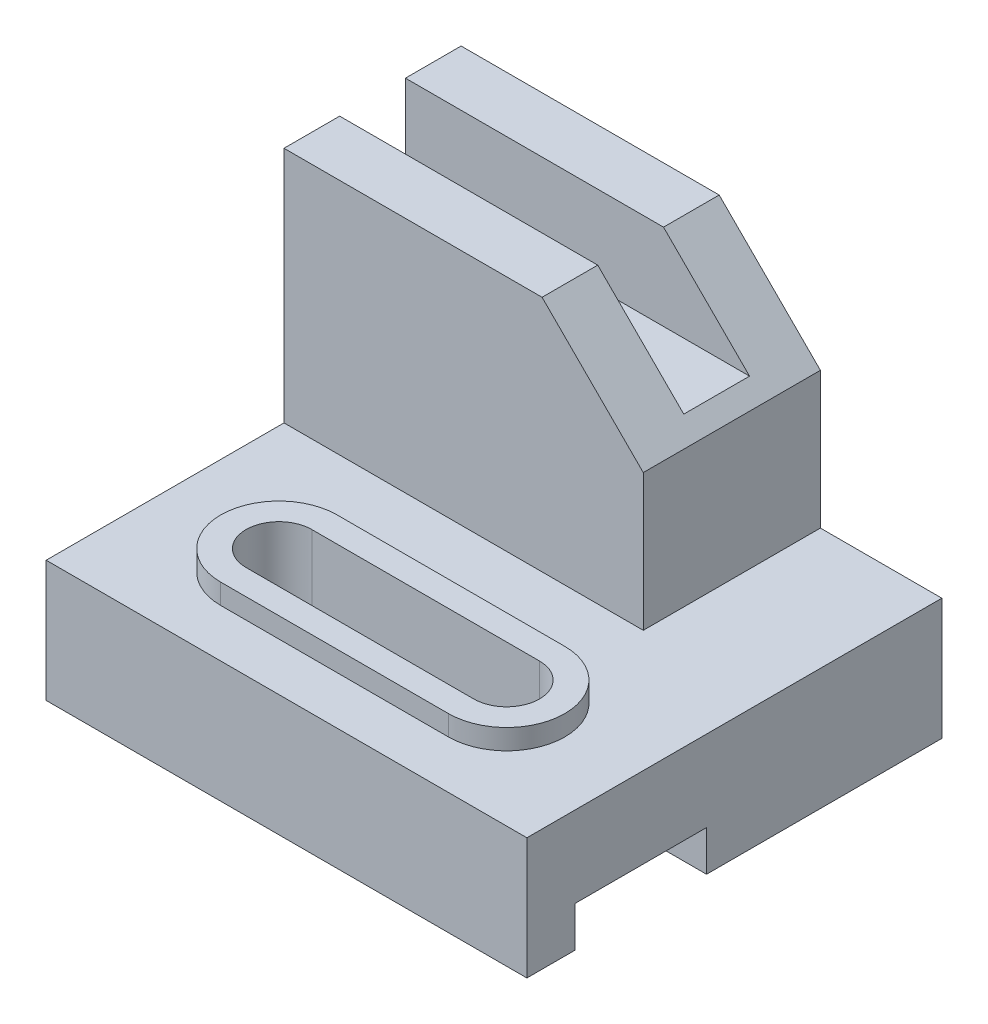
ISO-10303-21;
HEADER;
FILE_DESCRIPTION(('STEP AP214'),'2;1');
FILE_NAME('part.step','',(''),(''),'','','');
FILE_SCHEMA(('AUTOMOTIVE_DESIGN { 1 0 10303 214 1 1 1 1 }'));
ENDSEC;
DATA;
#1=APPLICATION_CONTEXT('core data for automotive mechanical design processes');
#2=APPLICATION_PROTOCOL_DEFINITION('international standard','automotive_design',2000,#1);
#3=PRODUCT_CONTEXT('',#1,'mechanical');
#4=PRODUCT('Part','Part','',(#3));
#5=PRODUCT_RELATED_PRODUCT_CATEGORY('part','',(#4));
#6=PRODUCT_DEFINITION_FORMATION('','',#4);
#7=PRODUCT_DEFINITION_CONTEXT('part definition',#1,'design');
#8=PRODUCT_DEFINITION('design','',#6,#7);
#9=PRODUCT_DEFINITION_SHAPE('','',#8);
#10=(LENGTH_UNIT() NAMED_UNIT(*) SI_UNIT(.MILLI.,.METRE.));
#11=(NAMED_UNIT(*) PLANE_ANGLE_UNIT() SI_UNIT($,.RADIAN.));
#12=(NAMED_UNIT(*) SI_UNIT($,.STERADIAN.) SOLID_ANGLE_UNIT());
#13=UNCERTAINTY_MEASURE_WITH_UNIT(LENGTH_MEASURE(1.E-05),#10,'distance_accuracy_value','');
#14=(GEOMETRIC_REPRESENTATION_CONTEXT(3) GLOBAL_UNCERTAINTY_ASSIGNED_CONTEXT((#13)) GLOBAL_UNIT_ASSIGNED_CONTEXT((#10,
#11,#12)) REPRESENTATION_CONTEXT('',''));
#15=CARTESIAN_POINT('',(0.,0.,0.));
#16=DIRECTION('',(0.,0.,1.));
#17=DIRECTION('',(1.,0.,0.));
#18=AXIS2_PLACEMENT_3D('',#15,#16,#17);
#19=CARTESIAN_POINT('',(95.,24.,0.));
#20=DIRECTION('',(0.,1.,0.));
#21=DIRECTION('',(0.,0.,1.));
#22=AXIS2_PLACEMENT_3D('',#19,#20,#21);
#23=PLANE('',#22);
#24=DIRECTION('',(0.,0.,-1.));
#25=VECTOR('',#24,1.);
#26=CARTESIAN_POINT('',(71.,24.,0.));
#27=LINE('',#26,#25);
#28=CARTESIAN_POINT('',(71.,24.,-47.));
#29=VERTEX_POINT('',#28);
#30=CARTESIAN_POINT('',(71.,24.,-82.));
#31=VERTEX_POINT('',#30);
#32=EDGE_CURVE('E345',#29,#31,#27,.T.);
#33=ORIENTED_EDGE('',*,*,#32,.F.);
#34=DIRECTION('',(-1.,0.,0.));
#35=VECTOR('',#34,1.);
#36=CARTESIAN_POINT('',(71.,24.,-47.));
#37=LINE('',#36,#35);
#38=CARTESIAN_POINT('',(0.,24.,-47.));
#39=VERTEX_POINT('',#38);
#40=EDGE_CURVE('E316',#29,#39,#37,.T.);
#41=ORIENTED_EDGE('',*,*,#40,.T.);
#42=DIRECTION('',(0.,0.,-1.));
#43=VECTOR('',#42,1.);
#44=CARTESIAN_POINT('',(0.,24.,0.));
#45=LINE('',#44,#43);
#46=CARTESIAN_POINT('',(0.,24.,0.));
#47=VERTEX_POINT('',#46);
#48=EDGE_CURVE('E279',#47,#39,#45,.T.);
#49=ORIENTED_EDGE('',*,*,#48,.F.);
#50=DIRECTION('',(-1.,0.,0.));
#51=VECTOR('',#50,1.);
#52=CARTESIAN_POINT('',(95.,24.,0.));
#53=LINE('',#52,#51);
#54=CARTESIAN_POINT('',(95.,24.,0.));
#55=VERTEX_POINT('',#54);
#56=EDGE_CURVE('E255',#55,#47,#53,.T.);
#57=ORIENTED_EDGE('',*,*,#56,.F.);
#58=DIRECTION('',(0.,0.,-1.));
#59=VECTOR('',#58,1.);
#60=CARTESIAN_POINT('',(95.,24.,0.));
#61=LINE('',#60,#59);
#62=CARTESIAN_POINT('',(95.,24.,-82.));
#63=VERTEX_POINT('',#62);
#64=EDGE_CURVE('E300',#55,#63,#61,.T.);
#65=ORIENTED_EDGE('',*,*,#64,.T.);
#66=DIRECTION('',(-1.,0.,0.));
#67=VECTOR('',#66,1.);
#68=CARTESIAN_POINT('',(95.,24.,-82.));
#69=LINE('',#68,#67);
#70=EDGE_CURVE('E253',#63,#31,#69,.T.);
#71=ORIENTED_EDGE('',*,*,#70,.T.);
#72=EDGE_LOOP('',(#33,#41,#49,#57,#65,#71));
#73=FACE_BOUND('',#72,.T.);
#74=DIRECTION('',(1.,0.,0.));
#75=VECTOR('',#74,1.);
#76=CARTESIAN_POINT('',(25.,24.,-9.5));
#77=LINE('',#76,#75);
#78=CARTESIAN_POINT('',(25.,24.,-9.5));
#79=VERTEX_POINT('',#78);
#80=CARTESIAN_POINT('',(70.,24.,-9.5));
#81=VERTEX_POINT('',#80);
#82=EDGE_CURVE('E362',#79,#81,#77,.T.);
#83=ORIENTED_EDGE('',*,*,#82,.F.);
#84=CARTESIAN_POINT('',(25.,24.,-21.));
#85=DIRECTION('',(0.,1.,0.));
#86=DIRECTION('',(0.,0.,1.));
#87=AXIS2_PLACEMENT_3D('',#84,#85,#86);
#88=CIRCLE('',#87,11.5);
#89=CARTESIAN_POINT('',(25.,24.,-32.5));
#90=VERTEX_POINT('',#89);
#91=EDGE_CURVE('E212',#90,#79,#88,.T.);
#92=ORIENTED_EDGE('',*,*,#91,.F.);
#93=DIRECTION('',(-1.,0.,0.));
#94=VECTOR('',#93,1.);
#95=CARTESIAN_POINT('',(25.,24.,-32.5));
#96=LINE('',#95,#94);
#97=CARTESIAN_POINT('',(70.,24.,-32.5));
#98=VERTEX_POINT('',#97);
#99=EDGE_CURVE('E359',#98,#90,#96,.T.);
#100=ORIENTED_EDGE('',*,*,#99,.F.);
#101=CARTESIAN_POINT('',(70.,24.,-21.));
#102=DIRECTION('',(0.,1.,0.));
#103=DIRECTION('',(0.,0.,1.));
#104=AXIS2_PLACEMENT_3D('',#101,#102,#103);
#105=CIRCLE('',#104,11.5);
#106=EDGE_CURVE('E356',#81,#98,#105,.T.);
#107=ORIENTED_EDGE('',*,*,#106,.F.);
#108=EDGE_LOOP('',(#83,#92,#100,#107));
#109=FACE_BOUND('',#108,.T.);
#110=ADVANCED_FACE('F43',(#73,#109),#23,.T.);
#111=CARTESIAN_POINT('',(95.,0.,-35.5));
#112=DIRECTION('',(0.,0.,1.));
#113=DIRECTION('',(1.,0.,0.));
#114=AXIS2_PLACEMENT_3D('',#111,#112,#113);
#115=PLANE('',#114);
#116=DIRECTION('',(0.,1.,0.));
#117=VECTOR('',#116,1.);
#118=CARTESIAN_POINT('',(0.,0.,-35.5));
#119=LINE('',#118,#117);
#120=CARTESIAN_POINT('',(0.,0.,-35.5));
#121=VERTEX_POINT('',#120);
#122=CARTESIAN_POINT('',(0.,8.,-35.5));
#123=VERTEX_POINT('',#122);
#124=EDGE_CURVE('E288',#121,#123,#119,.T.);
#125=ORIENTED_EDGE('',*,*,#124,.F.);
#126=DIRECTION('',(-1.,0.,0.));
#127=VECTOR('',#126,1.);
#128=CARTESIAN_POINT('',(95.,0.,-35.5));
#129=LINE('',#128,#127);
#130=CARTESIAN_POINT('',(95.,0.,-35.5));
#131=VERTEX_POINT('',#130);
#132=EDGE_CURVE('E248',#131,#121,#129,.T.);
#133=ORIENTED_EDGE('',*,*,#132,.F.);
#134=DIRECTION('',(0.,1.,0.));
#135=VECTOR('',#134,1.);
#136=CARTESIAN_POINT('',(95.,0.,-35.5));
#137=LINE('',#136,#135);
#138=CARTESIAN_POINT('',(95.,8.,-35.5));
#139=VERTEX_POINT('',#138);
#140=EDGE_CURVE('E269',#131,#139,#137,.T.);
#141=ORIENTED_EDGE('',*,*,#140,.T.);
#142=DIRECTION('',(-1.,0.,0.));
#143=VECTOR('',#142,1.);
#144=CARTESIAN_POINT('',(95.,8.,-35.5));
#145=LINE('',#144,#143);
#146=EDGE_CURVE('E262',#139,#123,#145,.T.);
#147=ORIENTED_EDGE('',*,*,#146,.T.);
#148=EDGE_LOOP('',(#125,#133,#141,#147));
#149=FACE_BOUND('',#148,.T.);
#150=ADVANCED_FACE('F400',(#149),#115,.T.);
#151=CARTESIAN_POINT('',(95.,0.,0.));
#152=DIRECTION('',(0.,1.,0.));
#153=DIRECTION('',(0.,0.,1.));
#154=AXIS2_PLACEMENT_3D('',#151,#152,#153);
#155=PLANE('',#154);
#156=DIRECTION('',(0.,0.,-1.));
#157=VECTOR('',#156,1.);
#158=CARTESIAN_POINT('',(0.,0.,0.));
#159=LINE('',#158,#157);
#160=CARTESIAN_POINT('',(0.,0.,-82.));
#161=VERTEX_POINT('',#160);
#162=EDGE_CURVE('E281',#121,#161,#159,.T.);
#163=ORIENTED_EDGE('',*,*,#162,.T.);
#164=DIRECTION('',(-1.,0.,0.));
#165=VECTOR('',#164,1.);
#166=CARTESIAN_POINT('',(95.,0.,-82.));
#167=LINE('',#166,#165);
#168=CARTESIAN_POINT('',(95.,0.,-82.));
#169=VERTEX_POINT('',#168);
#170=EDGE_CURVE('E247',#169,#161,#167,.T.);
#171=ORIENTED_EDGE('',*,*,#170,.F.);
#172=DIRECTION('',(0.,0.,-1.));
#173=VECTOR('',#172,1.);
#174=CARTESIAN_POINT('',(95.,0.,0.));
#175=LINE('',#174,#173);
#176=EDGE_CURVE('E302',#131,#169,#175,.T.);
#177=ORIENTED_EDGE('',*,*,#176,.F.);
#178=ORIENTED_EDGE('',*,*,#132,.T.);
#179=EDGE_LOOP('',(#163,#171,#177,#178));
#180=FACE_BOUND('',#179,.T.);
#181=ADVANCED_FACE('F409',(#180),#155,.F.);
#182=CARTESIAN_POINT('',(95.,0.,-82.));
#183=DIRECTION('',(0.,0.,1.));
#184=DIRECTION('',(1.,0.,0.));
#185=AXIS2_PLACEMENT_3D('',#182,#183,#184);
#186=PLANE('',#185);
#187=DIRECTION('',(-1.,0.,0.));
#188=VECTOR('',#187,1.);
#189=CARTESIAN_POINT('',(71.,71.,-82.));
#190=LINE('',#189,#188);
#191=CARTESIAN_POINT('',(50.9999999999999,71.,-82.));
#192=VERTEX_POINT('',#191);
#193=CARTESIAN_POINT('',(0.,71.,-82.));
#194=VERTEX_POINT('',#193);
#195=EDGE_CURVE('E317',#192,#194,#190,.T.);
#196=ORIENTED_EDGE('',*,*,#195,.F.);
#197=DIRECTION('',(0.707106781186548,-0.707106781186547,0.));
#198=VECTOR('',#197,1.);
#199=CARTESIAN_POINT('',(71.,51.,-82.));
#200=LINE('',#199,#198);
#201=CARTESIAN_POINT('',(71.,51.,-82.));
#202=VERTEX_POINT('',#201);
#203=EDGE_CURVE('E231',#192,#202,#200,.T.);
#204=ORIENTED_EDGE('',*,*,#203,.T.);
#205=DIRECTION('',(0.,1.,0.));
#206=VECTOR('',#205,1.);
#207=CARTESIAN_POINT('',(71.,0.,-82.));
#208=LINE('',#207,#206);
#209=EDGE_CURVE('E321',#31,#202,#208,.T.);
#210=ORIENTED_EDGE('',*,*,#209,.F.);
#211=ORIENTED_EDGE('',*,*,#70,.F.);
#212=DIRECTION('',(0.,1.,0.));
#213=VECTOR('',#212,1.);
#214=CARTESIAN_POINT('',(95.,0.,-82.));
#215=LINE('',#214,#213);
#216=EDGE_CURVE('E303',#169,#63,#215,.T.);
#217=ORIENTED_EDGE('',*,*,#216,.F.);
#218=ORIENTED_EDGE('',*,*,#170,.T.);
#219=DIRECTION('',(0.,1.,0.));
#220=VECTOR('',#219,1.);
#221=CARTESIAN_POINT('',(0.,0.,-82.));
#222=LINE('',#221,#220);
#223=EDGE_CURVE('E282',#161,#194,#222,.T.);
#224=ORIENTED_EDGE('',*,*,#223,.T.);
#225=EDGE_LOOP('',(#196,#204,#210,#211,#217,#218,#224));
#226=FACE_BOUND('',#225,.T.);
#227=ADVANCED_FACE('F411',(#226),#186,.F.);
#228=CARTESIAN_POINT('',(95.,0.,0.));
#229=DIRECTION('',(0.,0.,1.));
#230=DIRECTION('',(1.,0.,0.));
#231=AXIS2_PLACEMENT_3D('',#228,#229,#230);
#232=PLANE('',#231);
#233=DIRECTION('',(0.,1.,0.));
#234=VECTOR('',#233,1.);
#235=CARTESIAN_POINT('',(0.,0.,0.));
#236=LINE('',#235,#234);
#237=CARTESIAN_POINT('',(0.,0.,0.));
#238=VERTEX_POINT('',#237);
#239=EDGE_CURVE('E274',#238,#47,#236,.T.);
#240=ORIENTED_EDGE('',*,*,#239,.F.);
#241=DIRECTION('',(-1.,0.,0.));
#242=VECTOR('',#241,1.);
#243=CARTESIAN_POINT('',(95.,0.,0.));
#244=LINE('',#243,#242);
#245=CARTESIAN_POINT('',(95.,0.,0.));
#246=VERTEX_POINT('',#245);
#247=EDGE_CURVE('E258',#246,#238,#244,.T.);
#248=ORIENTED_EDGE('',*,*,#247,.F.);
#249=DIRECTION('',(0.,1.,0.));
#250=VECTOR('',#249,1.);
#251=CARTESIAN_POINT('',(95.,0.,0.));
#252=LINE('',#251,#250);
#253=EDGE_CURVE('E293',#246,#55,#252,.T.);
#254=ORIENTED_EDGE('',*,*,#253,.T.);
#255=ORIENTED_EDGE('',*,*,#56,.T.);
#256=EDGE_LOOP('',(#240,#248,#254,#255));
#257=FACE_BOUND('',#256,.T.);
#258=ADVANCED_FACE('F412',(#257),#232,.T.);
#259=CARTESIAN_POINT('',(95.,0.,0.));
#260=DIRECTION('',(0.,1.,0.));
#261=DIRECTION('',(0.,0.,1.));
#262=AXIS2_PLACEMENT_3D('',#259,#260,#261);
#263=PLANE('',#262);
#264=DIRECTION('',(0.,0.,-1.));
#265=VECTOR('',#264,1.);
#266=CARTESIAN_POINT('',(0.,0.,0.));
#267=LINE('',#266,#265);
#268=CARTESIAN_POINT('',(0.,0.,-9.5));
#269=VERTEX_POINT('',#268);
#270=EDGE_CURVE('E272',#238,#269,#267,.T.);
#271=ORIENTED_EDGE('',*,*,#270,.T.);
#272=DIRECTION('',(-1.,0.,0.));
#273=VECTOR('',#272,1.);
#274=CARTESIAN_POINT('',(95.,0.,-9.5));
#275=LINE('',#274,#273);
#276=CARTESIAN_POINT('',(95.,0.,-9.5));
#277=VERTEX_POINT('',#276);
#278=EDGE_CURVE('E256',#277,#269,#275,.T.);
#279=ORIENTED_EDGE('',*,*,#278,.F.);
#280=DIRECTION('',(0.,0.,-1.));
#281=VECTOR('',#280,1.);
#282=CARTESIAN_POINT('',(95.,0.,0.));
#283=LINE('',#282,#281);
#284=EDGE_CURVE('E291',#246,#277,#283,.T.);
#285=ORIENTED_EDGE('',*,*,#284,.F.);
#286=ORIENTED_EDGE('',*,*,#247,.T.);
#287=EDGE_LOOP('',(#271,#279,#285,#286));
#288=FACE_BOUND('',#287,.T.);
#289=ADVANCED_FACE('F471',(#288),#263,.F.);
#290=CARTESIAN_POINT('',(95.,0.,-9.5));
#291=DIRECTION('',(0.,0.,1.));
#292=DIRECTION('',(1.,0.,0.));
#293=AXIS2_PLACEMENT_3D('',#290,#291,#292);
#294=PLANE('',#293);
#295=DIRECTION('',(0.,1.,0.));
#296=VECTOR('',#295,1.);
#297=CARTESIAN_POINT('',(0.,0.,-9.5));
#298=LINE('',#297,#296);
#299=CARTESIAN_POINT('',(0.,8.,-9.5));
#300=VERTEX_POINT('',#299);
#301=EDGE_CURVE('E271',#269,#300,#298,.T.);
#302=ORIENTED_EDGE('',*,*,#301,.T.);
#303=DIRECTION('',(-1.,0.,0.));
#304=VECTOR('',#303,1.);
#305=CARTESIAN_POINT('',(95.,8.,-9.5));
#306=LINE('',#305,#304);
#307=CARTESIAN_POINT('',(95.,8.,-9.5));
#308=VERTEX_POINT('',#307);
#309=EDGE_CURVE('E261',#308,#300,#306,.T.);
#310=ORIENTED_EDGE('',*,*,#309,.F.);
#311=DIRECTION('',(0.,1.,0.));
#312=VECTOR('',#311,1.);
#313=CARTESIAN_POINT('',(95.,0.,-9.5));
#314=LINE('',#313,#312);
#315=EDGE_CURVE('E292',#277,#308,#314,.T.);
#316=ORIENTED_EDGE('',*,*,#315,.F.);
#317=ORIENTED_EDGE('',*,*,#278,.T.);
#318=EDGE_LOOP('',(#302,#310,#316,#317));
#319=FACE_BOUND('',#318,.T.);
#320=ADVANCED_FACE('F466',(#319),#294,.F.);
#321=CARTESIAN_POINT('',(95.,8.,0.));
#322=DIRECTION('',(0.,1.,0.));
#323=DIRECTION('',(0.,0.,1.));
#324=AXIS2_PLACEMENT_3D('',#321,#322,#323);
#325=PLANE('',#324);
#326=DIRECTION('',(-1.,0.,0.));
#327=VECTOR('',#326,1.);
#328=CARTESIAN_POINT('',(95.,8.,-27.5));
#329=LINE('',#328,#327);
#330=CARTESIAN_POINT('',(70.,8.00000000000001,-27.5));
#331=VERTEX_POINT('',#330);
#332=CARTESIAN_POINT('',(25.,8.00000000000001,-27.5));
#333=VERTEX_POINT('',#332);
#334=EDGE_CURVE('E55',#331,#333,#329,.T.);
#335=ORIENTED_EDGE('',*,*,#334,.T.);
#336=CARTESIAN_POINT('',(25.,8.00000000000001,-21.));
#337=DIRECTION('',(0.,1.,0.));
#338=DIRECTION('',(0.,0.,1.));
#339=AXIS2_PLACEMENT_3D('',#336,#337,#338);
#340=CIRCLE('',#339,6.5);
#341=CARTESIAN_POINT('',(25.,8.00000000000001,-14.5));
#342=VERTEX_POINT('',#341);
#343=EDGE_CURVE('E11',#333,#342,#340,.T.);
#344=ORIENTED_EDGE('',*,*,#343,.T.);
#345=DIRECTION('',(1.,0.,0.));
#346=VECTOR('',#345,1.);
#347=CARTESIAN_POINT('',(95.,8.,-14.5));
#348=LINE('',#347,#346);
#349=CARTESIAN_POINT('',(70.,8.,-14.5));
#350=VERTEX_POINT('',#349);
#351=EDGE_CURVE('E220',#342,#350,#348,.T.);
#352=ORIENTED_EDGE('',*,*,#351,.T.);
#353=CARTESIAN_POINT('',(70.,8.00000000000001,-21.));
#354=DIRECTION('',(0.,1.,0.));
#355=DIRECTION('',(0.,0.,1.));
#356=AXIS2_PLACEMENT_3D('',#353,#354,#355);
#357=CIRCLE('',#356,6.5);
#358=EDGE_CURVE('E222',#350,#331,#357,.T.);
#359=ORIENTED_EDGE('',*,*,#358,.T.);
#360=EDGE_LOOP('',(#335,#344,#352,#359));
#361=FACE_BOUND('',#360,.T.);
#362=DIRECTION('',(0.,0.,-1.));
#363=VECTOR('',#362,1.);
#364=CARTESIAN_POINT('',(0.,8.,0.));
#365=LINE('',#364,#363);
#366=EDGE_CURVE('E270',#300,#123,#365,.T.);
#367=ORIENTED_EDGE('',*,*,#366,.T.);
#368=ORIENTED_EDGE('',*,*,#146,.F.);
#369=DIRECTION('',(0.,0.,-1.));
#370=VECTOR('',#369,1.);
#371=CARTESIAN_POINT('',(95.,8.,0.));
#372=LINE('',#371,#370);
#373=EDGE_CURVE('E266',#308,#139,#372,.T.);
#374=ORIENTED_EDGE('',*,*,#373,.F.);
#375=ORIENTED_EDGE('',*,*,#309,.T.);
#376=EDGE_LOOP('',(#367,#368,#374,#375));
#377=FACE_BOUND('',#376,.T.);
#378=ADVANCED_FACE('F221',(#361,#377),#325,.F.);
#379=CARTESIAN_POINT('',(95.,0.,0.));
#380=DIRECTION('',(1.,0.,0.));
#381=DIRECTION('',(0.,0.,-1.));
#382=AXIS2_PLACEMENT_3D('',#379,#380,#381);
#383=PLANE('',#382);
#384=ORIENTED_EDGE('',*,*,#140,.F.);
#385=ORIENTED_EDGE('',*,*,#176,.T.);
#386=ORIENTED_EDGE('',*,*,#216,.T.);
#387=ORIENTED_EDGE('',*,*,#64,.F.);
#388=ORIENTED_EDGE('',*,*,#253,.F.);
#389=ORIENTED_EDGE('',*,*,#284,.T.);
#390=ORIENTED_EDGE('',*,*,#315,.T.);
#391=ORIENTED_EDGE('',*,*,#373,.T.);
#392=EDGE_LOOP('',(#384,#385,#386,#387,#388,#389,#390,#391));
#393=FACE_BOUND('',#392,.T.);
#394=ADVANCED_FACE('F465',(#393),#383,.T.);
#395=CARTESIAN_POINT('',(0.,0.,0.));
#396=DIRECTION('',(1.,0.,0.));
#397=DIRECTION('',(0.,0.,-1.));
#398=AXIS2_PLACEMENT_3D('',#395,#396,#397);
#399=PLANE('',#398);
#400=ORIENTED_EDGE('',*,*,#124,.T.);
#401=ORIENTED_EDGE('',*,*,#366,.F.);
#402=ORIENTED_EDGE('',*,*,#301,.F.);
#403=ORIENTED_EDGE('',*,*,#270,.F.);
#404=ORIENTED_EDGE('',*,*,#239,.T.);
#405=ORIENTED_EDGE('',*,*,#48,.T.);
#406=DIRECTION('',(0.,1.,0.));
#407=VECTOR('',#406,1.);
#408=CARTESIAN_POINT('',(0.,0.,-47.));
#409=LINE('',#408,#407);
#410=CARTESIAN_POINT('',(0.,71.,-47.));
#411=VERTEX_POINT('',#410);
#412=EDGE_CURVE('E325',#39,#411,#409,.T.);
#413=ORIENTED_EDGE('',*,*,#412,.T.);
#414=DIRECTION('',(0.,0.,1.));
#415=VECTOR('',#414,1.);
#416=CARTESIAN_POINT('',(0.,71.,0.));
#417=LINE('',#416,#415);
#418=CARTESIAN_POINT('',(0.,71.,-58.));
#419=VERTEX_POINT('',#418);
#420=EDGE_CURVE('E326',#419,#411,#417,.T.);
#421=ORIENTED_EDGE('',*,*,#420,.F.);
#422=DIRECTION('',(0.,-1.,0.));
#423=VECTOR('',#422,1.);
#424=CARTESIAN_POINT('',(0.,0.,-58.));
#425=LINE('',#424,#423);
#426=CARTESIAN_POINT('',(0.,54.,-58.));
#427=VERTEX_POINT('',#426);
#428=EDGE_CURVE('E328',#419,#427,#425,.T.);
#429=ORIENTED_EDGE('',*,*,#428,.T.);
#430=DIRECTION('',(0.,0.,-1.));
#431=VECTOR('',#430,1.);
#432=CARTESIAN_POINT('',(0.,54.,0.));
#433=LINE('',#432,#431);
#434=CARTESIAN_POINT('',(0.,54.,-71.));
#435=VERTEX_POINT('',#434);
#436=EDGE_CURVE('E335',#427,#435,#433,.T.);
#437=ORIENTED_EDGE('',*,*,#436,.T.);
#438=DIRECTION('',(0.,-1.,0.));
#439=VECTOR('',#438,1.);
#440=CARTESIAN_POINT('',(0.,0.,-71.));
#441=LINE('',#440,#439);
#442=CARTESIAN_POINT('',(0.,71.,-71.));
#443=VERTEX_POINT('',#442);
#444=EDGE_CURVE('E333',#443,#435,#441,.T.);
#445=ORIENTED_EDGE('',*,*,#444,.F.);
#446=DIRECTION('',(0.,0.,1.));
#447=VECTOR('',#446,1.);
#448=CARTESIAN_POINT('',(0.,71.,0.));
#449=LINE('',#448,#447);
#450=EDGE_CURVE('E340',#194,#443,#449,.T.);
#451=ORIENTED_EDGE('',*,*,#450,.F.);
#452=ORIENTED_EDGE('',*,*,#223,.F.);
#453=ORIENTED_EDGE('',*,*,#162,.F.);
#454=EDGE_LOOP('',(#400,#401,#402,#403,#404,#405,#413,#421,#429,#437,#445,#451,#452,#453));
#455=FACE_BOUND('',#454,.T.);
#456=ADVANCED_FACE('F432',(#455),#399,.F.);
#457=CARTESIAN_POINT('',(71.,71.,0.));
#458=DIRECTION('',(0.,-1.,0.));
#459=DIRECTION('',(0.,0.,-1.));
#460=AXIS2_PLACEMENT_3D('',#457,#458,#459);
#461=PLANE('',#460);
#462=DIRECTION('',(-1.,0.,0.));
#463=VECTOR('',#462,1.);
#464=CARTESIAN_POINT('',(71.,71.,-71.));
#465=LINE('',#464,#463);
#466=CARTESIAN_POINT('',(50.9999999999999,71.,-71.));
#467=VERTEX_POINT('',#466);
#468=EDGE_CURVE('E290',#467,#443,#465,.T.);
#469=ORIENTED_EDGE('',*,*,#468,.F.);
#470=DIRECTION('',(0.,0.,-1.));
#471=VECTOR('',#470,1.);
#472=CARTESIAN_POINT('',(50.9999999999999,71.,-82.));
#473=LINE('',#472,#471);
#474=EDGE_CURVE('E236',#467,#192,#473,.T.);
#475=ORIENTED_EDGE('',*,*,#474,.T.);
#476=ORIENTED_EDGE('',*,*,#195,.T.);
#477=ORIENTED_EDGE('',*,*,#450,.T.);
#478=EDGE_LOOP('',(#469,#475,#476,#477));
#479=FACE_BOUND('',#478,.T.);
#480=ADVANCED_FACE('F437',(#479),#461,.F.);
#481=CARTESIAN_POINT('',(71.,0.,-71.));
#482=DIRECTION('',(0.,0.,-1.));
#483=DIRECTION('',(-1.,0.,0.));
#484=AXIS2_PLACEMENT_3D('',#481,#482,#483);
#485=PLANE('',#484);
#486=DIRECTION('',(-1.,0.,0.));
#487=VECTOR('',#486,1.);
#488=CARTESIAN_POINT('',(71.,54.,-71.));
#489=LINE('',#488,#487);
#490=CARTESIAN_POINT('',(68.,54.,-71.));
#491=VERTEX_POINT('',#490);
#492=EDGE_CURVE('E306',#491,#435,#489,.T.);
#493=ORIENTED_EDGE('',*,*,#492,.F.);
#494=DIRECTION('',(-0.707106781186548,0.707106781186547,0.));
#495=VECTOR('',#494,1.);
#496=CARTESIAN_POINT('',(71.,51.,-71.));
#497=LINE('',#496,#495);
#498=EDGE_CURVE('E238',#491,#467,#497,.T.);
#499=ORIENTED_EDGE('',*,*,#498,.T.);
#500=ORIENTED_EDGE('',*,*,#468,.T.);
#501=ORIENTED_EDGE('',*,*,#444,.T.);
#502=EDGE_LOOP('',(#493,#499,#500,#501));
#503=FACE_BOUND('',#502,.T.);
#504=ADVANCED_FACE('F488',(#503),#485,.F.);
#505=CARTESIAN_POINT('',(71.,54.,0.));
#506=DIRECTION('',(0.,1.,0.));
#507=DIRECTION('',(0.,0.,1.));
#508=AXIS2_PLACEMENT_3D('',#505,#506,#507);
#509=PLANE('',#508);
#510=DIRECTION('',(0.,0.,-1.));
#511=VECTOR('',#510,1.);
#512=CARTESIAN_POINT('',(68.,54.,0.));
#513=LINE('',#512,#511);
#514=CARTESIAN_POINT('',(68.,54.,-58.));
#515=VERTEX_POINT('',#514);
#516=EDGE_CURVE('E244',#515,#491,#513,.T.);
#517=ORIENTED_EDGE('',*,*,#516,.T.);
#518=ORIENTED_EDGE('',*,*,#492,.T.);
#519=ORIENTED_EDGE('',*,*,#436,.F.);
#520=DIRECTION('',(-1.,0.,0.));
#521=VECTOR('',#520,1.);
#522=CARTESIAN_POINT('',(71.,54.,-58.));
#523=LINE('',#522,#521);
#524=EDGE_CURVE('E309',#515,#427,#523,.T.);
#525=ORIENTED_EDGE('',*,*,#524,.F.);
#526=EDGE_LOOP('',(#517,#518,#519,#525));
#527=FACE_BOUND('',#526,.T.);
#528=ADVANCED_FACE('F491',(#527),#509,.T.);
#529=CARTESIAN_POINT('',(71.,0.,-58.));
#530=DIRECTION('',(0.,0.,-1.));
#531=DIRECTION('',(0.,1.,0.));
#532=AXIS2_PLACEMENT_3D('',#529,#530,#531);
#533=PLANE('',#532);
#534=DIRECTION('',(-1.,0.,0.));
#535=VECTOR('',#534,1.);
#536=CARTESIAN_POINT('',(71.,71.,-58.));
#537=LINE('',#536,#535);
#538=CARTESIAN_POINT('',(50.9999999999999,71.,-58.));
#539=VERTEX_POINT('',#538);
#540=EDGE_CURVE('E315',#539,#419,#537,.T.);
#541=ORIENTED_EDGE('',*,*,#540,.F.);
#542=DIRECTION('',(0.707106781186548,-0.707106781186547,0.));
#543=VECTOR('',#542,1.);
#544=CARTESIAN_POINT('',(96.5,25.5000000000001,-58.));
#545=LINE('',#544,#543);
#546=EDGE_CURVE('E225',#539,#515,#545,.T.);
#547=ORIENTED_EDGE('',*,*,#546,.T.);
#548=ORIENTED_EDGE('',*,*,#524,.T.);
#549=ORIENTED_EDGE('',*,*,#428,.F.);
#550=EDGE_LOOP('',(#541,#547,#548,#549));
#551=FACE_BOUND('',#550,.T.);
#552=ADVANCED_FACE('F494',(#551),#533,.T.);
#553=CARTESIAN_POINT('',(71.,71.,0.));
#554=DIRECTION('',(0.,-1.,0.));
#555=DIRECTION('',(0.,0.,-1.));
#556=AXIS2_PLACEMENT_3D('',#553,#554,#555);
#557=PLANE('',#556);
#558=DIRECTION('',(-1.,0.,0.));
#559=VECTOR('',#558,1.);
#560=CARTESIAN_POINT('',(71.,71.,-47.));
#561=LINE('',#560,#559);
#562=CARTESIAN_POINT('',(50.9999999999999,71.,-47.));
#563=VERTEX_POINT('',#562);
#564=EDGE_CURVE('E314',#563,#411,#561,.T.);
#565=ORIENTED_EDGE('',*,*,#564,.F.);
#566=DIRECTION('',(0.,0.,-1.));
#567=VECTOR('',#566,1.);
#568=CARTESIAN_POINT('',(50.9999999999999,71.,-58.));
#569=LINE('',#568,#567);
#570=EDGE_CURVE('E233',#563,#539,#569,.T.);
#571=ORIENTED_EDGE('',*,*,#570,.T.);
#572=ORIENTED_EDGE('',*,*,#540,.T.);
#573=ORIENTED_EDGE('',*,*,#420,.T.);
#574=EDGE_LOOP('',(#565,#571,#572,#573));
#575=FACE_BOUND('',#574,.T.);
#576=ADVANCED_FACE('F496',(#575),#557,.F.);
#577=CARTESIAN_POINT('',(71.,0.,-47.));
#578=DIRECTION('',(0.,0.,1.));
#579=DIRECTION('',(1.,0.,0.));
#580=AXIS2_PLACEMENT_3D('',#577,#578,#579);
#581=PLANE('',#580);
#582=DIRECTION('',(0.,1.,0.));
#583=VECTOR('',#582,1.);
#584=CARTESIAN_POINT('',(71.,0.,-47.));
#585=LINE('',#584,#583);
#586=CARTESIAN_POINT('',(71.,51.,-47.));
#587=VERTEX_POINT('',#586);
#588=EDGE_CURVE('E324',#29,#587,#585,.T.);
#589=ORIENTED_EDGE('',*,*,#588,.T.);
#590=DIRECTION('',(-0.707106781186548,0.707106781186547,0.));
#591=VECTOR('',#590,1.);
#592=CARTESIAN_POINT('',(96.5,25.5000000000001,-47.));
#593=LINE('',#592,#591);
#594=EDGE_CURVE('E232',#587,#563,#593,.T.);
#595=ORIENTED_EDGE('',*,*,#594,.T.);
#596=ORIENTED_EDGE('',*,*,#564,.T.);
#597=ORIENTED_EDGE('',*,*,#412,.F.);
#598=ORIENTED_EDGE('',*,*,#40,.F.);
#599=EDGE_LOOP('',(#589,#595,#596,#597,#598));
#600=FACE_BOUND('',#599,.T.);
#601=ADVANCED_FACE('F448',(#600),#581,.T.);
#602=CARTESIAN_POINT('',(71.,0.,0.));
#603=DIRECTION('',(1.,0.,0.));
#604=DIRECTION('',(0.,0.,-1.));
#605=AXIS2_PLACEMENT_3D('',#602,#603,#604);
#606=PLANE('',#605);
#607=ORIENTED_EDGE('',*,*,#209,.T.);
#608=DIRECTION('',(0.,0.,1.));
#609=VECTOR('',#608,1.);
#610=CARTESIAN_POINT('',(71.,51.,-47.));
#611=LINE('',#610,#609);
#612=EDGE_CURVE('E241',#202,#587,#611,.T.);
#613=ORIENTED_EDGE('',*,*,#612,.T.);
#614=ORIENTED_EDGE('',*,*,#588,.F.);
#615=ORIENTED_EDGE('',*,*,#32,.T.);
#616=EDGE_LOOP('',(#607,#613,#614,#615));
#617=FACE_BOUND('',#616,.T.);
#618=ADVANCED_FACE('F450',(#617),#606,.T.);
#619=CARTESIAN_POINT('',(71.,51.,0.));
#620=DIRECTION('',(0.707106781186547,0.707106781186548,0.));
#621=DIRECTION('',(0.,0.,-1.));
#622=AXIS2_PLACEMENT_3D('',#619,#620,#621);
#623=PLANE('',#622);
#624=ORIENTED_EDGE('',*,*,#594,.F.);
#625=ORIENTED_EDGE('',*,*,#612,.F.);
#626=ORIENTED_EDGE('',*,*,#203,.F.);
#627=ORIENTED_EDGE('',*,*,#474,.F.);
#628=ORIENTED_EDGE('',*,*,#498,.F.);
#629=ORIENTED_EDGE('',*,*,#516,.F.);
#630=ORIENTED_EDGE('',*,*,#546,.F.);
#631=ORIENTED_EDGE('',*,*,#570,.F.);
#632=EDGE_LOOP('',(#624,#625,#626,#627,#628,#629,#630,#631));
#633=FACE_BOUND('',#632,.T.);
#634=ADVANCED_FACE('F46',(#633),#623,.T.);
#635=CARTESIAN_POINT('',(25.,28.,-21.));
#636=DIRECTION('',(0.,1.,0.));
#637=DIRECTION('',(0.,0.,1.));
#638=AXIS2_PLACEMENT_3D('',#635,#636,#637);
#639=PLANE('',#638);
#640=CARTESIAN_POINT('',(25.,28.,-21.));
#641=DIRECTION('',(0.,1.,0.));
#642=DIRECTION('',(0.,0.,1.));
#643=AXIS2_PLACEMENT_3D('',#640,#641,#642);
#644=CIRCLE('',#643,11.5);
#645=CARTESIAN_POINT('',(25.,28.,-32.5));
#646=VERTEX_POINT('',#645);
#647=CARTESIAN_POINT('',(25.,28.,-9.5));
#648=VERTEX_POINT('',#647);
#649=EDGE_CURVE('E360',#646,#648,#644,.T.);
#650=ORIENTED_EDGE('',*,*,#649,.T.);
#651=DIRECTION('',(1.,0.,0.));
#652=VECTOR('',#651,1.);
#653=CARTESIAN_POINT('',(25.,28.,-9.5));
#654=LINE('',#653,#652);
#655=CARTESIAN_POINT('',(70.,28.,-9.5));
#656=VERTEX_POINT('',#655);
#657=EDGE_CURVE('E369',#648,#656,#654,.T.);
#658=ORIENTED_EDGE('',*,*,#657,.T.);
#659=CARTESIAN_POINT('',(70.,28.,-21.));
#660=DIRECTION('',(0.,1.,0.));
#661=DIRECTION('',(0.,0.,1.));
#662=AXIS2_PLACEMENT_3D('',#659,#660,#661);
#663=CIRCLE('',#662,11.5);
#664=CARTESIAN_POINT('',(70.,28.,-32.5));
#665=VERTEX_POINT('',#664);
#666=EDGE_CURVE('E370',#656,#665,#663,.T.);
#667=ORIENTED_EDGE('',*,*,#666,.T.);
#668=DIRECTION('',(-1.,0.,0.));
#669=VECTOR('',#668,1.);
#670=CARTESIAN_POINT('',(25.,28.,-32.5));
#671=LINE('',#670,#669);
#672=EDGE_CURVE('E358',#665,#646,#671,.T.);
#673=ORIENTED_EDGE('',*,*,#672,.T.);
#674=EDGE_LOOP('',(#650,#658,#667,#673));
#675=FACE_BOUND('',#674,.T.);
#676=DIRECTION('',(1.,0.,0.));
#677=VECTOR('',#676,1.);
#678=CARTESIAN_POINT('',(25.,28.,-14.5));
#679=LINE('',#678,#677);
#680=CARTESIAN_POINT('',(25.,28.,-14.5));
#681=VERTEX_POINT('',#680);
#682=CARTESIAN_POINT('',(70.,28.,-14.5));
#683=VERTEX_POINT('',#682);
#684=EDGE_CURVE('E382',#681,#683,#679,.T.);
#685=ORIENTED_EDGE('',*,*,#684,.F.);
#686=CARTESIAN_POINT('',(25.,28.,-21.));
#687=DIRECTION('',(0.,1.,0.));
#688=DIRECTION('',(0.,0.,1.));
#689=AXIS2_PLACEMENT_3D('',#686,#687,#688);
#690=CIRCLE('',#689,6.5);
#691=CARTESIAN_POINT('',(25.,28.,-27.5));
#692=VERTEX_POINT('',#691);
#693=EDGE_CURVE('E215',#692,#681,#690,.T.);
#694=ORIENTED_EDGE('',*,*,#693,.F.);
#695=DIRECTION('',(-1.,0.,0.));
#696=VECTOR('',#695,1.);
#697=CARTESIAN_POINT('',(25.,28.,-27.5));
#698=LINE('',#697,#696);
#699=CARTESIAN_POINT('',(70.,28.,-27.5));
#700=VERTEX_POINT('',#699);
#701=EDGE_CURVE('E378',#700,#692,#698,.T.);
#702=ORIENTED_EDGE('',*,*,#701,.F.);
#703=CARTESIAN_POINT('',(70.,28.,-21.));
#704=DIRECTION('',(0.,1.,0.));
#705=DIRECTION('',(0.,0.,1.));
#706=AXIS2_PLACEMENT_3D('',#703,#704,#705);
#707=CIRCLE('',#706,6.5);
#708=EDGE_CURVE('E379',#683,#700,#707,.T.);
#709=ORIENTED_EDGE('',*,*,#708,.F.);
#710=EDGE_LOOP('',(#685,#694,#702,#709));
#711=FACE_BOUND('',#710,.T.);
#712=ADVANCED_FACE('F388',(#675,#711),#639,.T.);
#713=CARTESIAN_POINT('',(25.,28.,-21.));
#714=DIRECTION('',(0.,-1.,0.));
#715=DIRECTION('',(0.,0.,-1.));
#716=AXIS2_PLACEMENT_3D('',#713,#714,#715);
#717=CYLINDRICAL_SURFACE('',#716,11.5);
#718=ORIENTED_EDGE('',*,*,#91,.T.);
#719=DIRECTION('',(0.,-1.,0.));
#720=VECTOR('',#719,1.);
#721=CARTESIAN_POINT('',(25.,28.,-9.5));
#722=LINE('',#721,#720);
#723=EDGE_CURVE('E343',#648,#79,#722,.T.);
#724=ORIENTED_EDGE('',*,*,#723,.F.);
#725=ORIENTED_EDGE('',*,*,#649,.F.);
#726=DIRECTION('',(0.,-1.,0.));
#727=VECTOR('',#726,1.);
#728=CARTESIAN_POINT('',(25.,28.,-32.5));
#729=LINE('',#728,#727);
#730=EDGE_CURVE('E355',#646,#90,#729,.T.);
#731=ORIENTED_EDGE('',*,*,#730,.T.);
#732=EDGE_LOOP('',(#718,#724,#725,#731));
#733=FACE_BOUND('',#732,.T.);
#734=ADVANCED_FACE('F507',(#733),#717,.T.);
#735=CARTESIAN_POINT('',(25.,28.,-9.5));
#736=DIRECTION('',(0.,0.,-1.));
#737=DIRECTION('',(-1.,0.,0.));
#738=AXIS2_PLACEMENT_3D('',#735,#736,#737);
#739=PLANE('',#738);
#740=ORIENTED_EDGE('',*,*,#82,.T.);
#741=DIRECTION('',(0.,-1.,0.));
#742=VECTOR('',#741,1.);
#743=CARTESIAN_POINT('',(70.,28.,-9.5));
#744=LINE('',#743,#742);
#745=EDGE_CURVE('E349',#656,#81,#744,.T.);
#746=ORIENTED_EDGE('',*,*,#745,.F.);
#747=ORIENTED_EDGE('',*,*,#657,.F.);
#748=ORIENTED_EDGE('',*,*,#723,.T.);
#749=EDGE_LOOP('',(#740,#746,#747,#748));
#750=FACE_BOUND('',#749,.T.);
#751=ADVANCED_FACE('F512',(#750),#739,.F.);
#752=CARTESIAN_POINT('',(70.,28.,-21.));
#753=DIRECTION('',(0.,-1.,0.));
#754=DIRECTION('',(0.,0.,-1.));
#755=AXIS2_PLACEMENT_3D('',#752,#753,#754);
#756=CYLINDRICAL_SURFACE('',#755,11.5);
#757=ORIENTED_EDGE('',*,*,#106,.T.);
#758=DIRECTION('',(0.,-1.,0.));
#759=VECTOR('',#758,1.);
#760=CARTESIAN_POINT('',(70.,28.,-32.5));
#761=LINE('',#760,#759);
#762=EDGE_CURVE('E69',#665,#98,#761,.T.);
#763=ORIENTED_EDGE('',*,*,#762,.F.);
#764=ORIENTED_EDGE('',*,*,#666,.F.);
#765=ORIENTED_EDGE('',*,*,#745,.T.);
#766=EDGE_LOOP('',(#757,#763,#764,#765));
#767=FACE_BOUND('',#766,.T.);
#768=ADVANCED_FACE('F513',(#767),#756,.T.);
#769=CARTESIAN_POINT('',(25.,28.,-32.5));
#770=DIRECTION('',(0.,0.,1.));
#771=DIRECTION('',(1.,0.,0.));
#772=AXIS2_PLACEMENT_3D('',#769,#770,#771);
#773=PLANE('',#772);
#774=ORIENTED_EDGE('',*,*,#99,.T.);
#775=ORIENTED_EDGE('',*,*,#730,.F.);
#776=ORIENTED_EDGE('',*,*,#672,.F.);
#777=ORIENTED_EDGE('',*,*,#762,.T.);
#778=EDGE_LOOP('',(#774,#775,#776,#777));
#779=FACE_BOUND('',#778,.T.);
#780=ADVANCED_FACE('F516',(#779),#773,.F.);
#781=CARTESIAN_POINT('',(25.,28.,-21.));
#782=DIRECTION('',(0.,-1.,0.));
#783=DIRECTION('',(0.,0.,-1.));
#784=AXIS2_PLACEMENT_3D('',#781,#782,#783);
#785=CYLINDRICAL_SURFACE('',#784,6.5);
#786=DIRECTION('',(0.,-1.,0.));
#787=VECTOR('',#786,1.);
#788=CARTESIAN_POINT('',(25.,28.,-14.5));
#789=LINE('',#788,#787);
#790=EDGE_CURVE('E210',#681,#342,#789,.T.);
#791=ORIENTED_EDGE('',*,*,#790,.T.);
#792=ORIENTED_EDGE('',*,*,#343,.F.);
#793=DIRECTION('',(0.,-1.,0.));
#794=VECTOR('',#793,1.);
#795=CARTESIAN_POINT('',(25.,28.,-27.5));
#796=LINE('',#795,#794);
#797=EDGE_CURVE('E376',#692,#333,#796,.T.);
#798=ORIENTED_EDGE('',*,*,#797,.F.);
#799=ORIENTED_EDGE('',*,*,#693,.T.);
#800=EDGE_LOOP('',(#791,#792,#798,#799));
#801=FACE_BOUND('',#800,.T.);
#802=ADVANCED_FACE('F208',(#801),#785,.F.);
#803=CARTESIAN_POINT('',(25.,28.,-14.5));
#804=DIRECTION('',(0.,0.,-1.));
#805=DIRECTION('',(-1.,0.,0.));
#806=AXIS2_PLACEMENT_3D('',#803,#804,#805);
#807=PLANE('',#806);
#808=DIRECTION('',(0.,-1.,0.));
#809=VECTOR('',#808,1.);
#810=CARTESIAN_POINT('',(70.,28.,-14.5));
#811=LINE('',#810,#809);
#812=EDGE_CURVE('E56',#683,#350,#811,.T.);
#813=ORIENTED_EDGE('',*,*,#812,.T.);
#814=ORIENTED_EDGE('',*,*,#351,.F.);
#815=ORIENTED_EDGE('',*,*,#790,.F.);
#816=ORIENTED_EDGE('',*,*,#684,.T.);
#817=EDGE_LOOP('',(#813,#814,#815,#816));
#818=FACE_BOUND('',#817,.T.);
#819=ADVANCED_FACE('F217',(#818),#807,.T.);
#820=CARTESIAN_POINT('',(70.,28.,-21.));
#821=DIRECTION('',(0.,-1.,0.));
#822=DIRECTION('',(0.,0.,-1.));
#823=AXIS2_PLACEMENT_3D('',#820,#821,#822);
#824=CYLINDRICAL_SURFACE('',#823,6.5);
#825=DIRECTION('',(0.,-1.,0.));
#826=VECTOR('',#825,1.);
#827=CARTESIAN_POINT('',(70.,28.,-27.5));
#828=LINE('',#827,#826);
#829=EDGE_CURVE('E372',#700,#331,#828,.T.);
#830=ORIENTED_EDGE('',*,*,#829,.T.);
#831=ORIENTED_EDGE('',*,*,#358,.F.);
#832=ORIENTED_EDGE('',*,*,#812,.F.);
#833=ORIENTED_EDGE('',*,*,#708,.T.);
#834=EDGE_LOOP('',(#830,#831,#832,#833));
#835=FACE_BOUND('',#834,.T.);
#836=ADVANCED_FACE('F389',(#835),#824,.F.);
#837=CARTESIAN_POINT('',(25.,28.,-27.5));
#838=DIRECTION('',(0.,0.,1.));
#839=DIRECTION('',(1.,0.,0.));
#840=AXIS2_PLACEMENT_3D('',#837,#838,#839);
#841=PLANE('',#840);
#842=ORIENTED_EDGE('',*,*,#797,.T.);
#843=ORIENTED_EDGE('',*,*,#334,.F.);
#844=ORIENTED_EDGE('',*,*,#829,.F.);
#845=ORIENTED_EDGE('',*,*,#701,.T.);
#846=EDGE_LOOP('',(#842,#843,#844,#845));
#847=FACE_BOUND('',#846,.T.);
#848=ADVANCED_FACE('F392',(#847),#841,.T.);
#849=CLOSED_SHELL('',(#110,#150,#181,#227,#258,#289,#320,#378,#394,#456,#480,#504,#528,#552,
#576,#601,#618,#634,#712,#734,#751,#768,#780,#802,#819,#836,#848));
#850=MANIFOLD_SOLID_BREP('B2',#849);
#851=ADVANCED_BREP_SHAPE_REPRESENTATION('',(#18,#850),#14);
#852=SHAPE_DEFINITION_REPRESENTATION(#9,#851);
ENDSEC;
END-ISO-10303-21;
